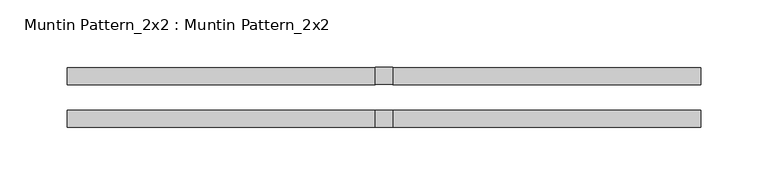
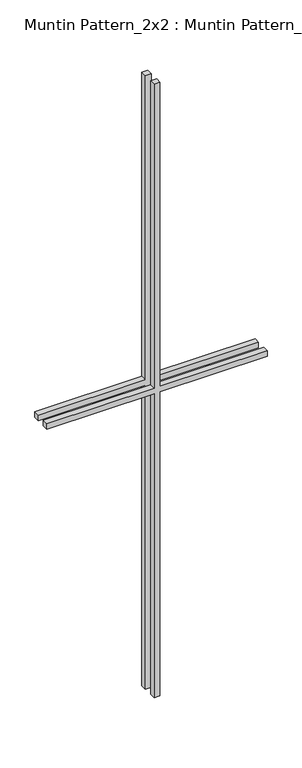
"""IFC4 building model written with IfcOpenShell, lengths in millimetres: proxy geometry, Muntin Pattern_2x2 : Muntin Pattern_2x2."""

from ifc_helpers import new_model, si_unit, frame, origin, place, context, project, spatial, polyline, outline, extrude, source, transform, mapped, element, save


def muntin_pattern_2x2_muntin_pattern_2x2_8031e6f6(model_context):
    return source(origin(), model_context, "Body", "SweptSolid", [
        extrude(outline(polyline([(698.5, -6.35), (698.5, -234.95), (685.8, -234.95), (685.8, -6.35), (0.0, -6.35), (0.0, 6.35), (685.8, 6.35), (685.8, 234.95), (698.5, 234.95), (698.5, 6.35), (1384.3, 6.35), (1384.3, -6.35), (698.5, -6.35)])), frame((0.0, 9.525, 0.0), z_axis=(0.0, 1.0, 0.0), x_axis=(0.0, 0.0, 1.0)), (0.0, 0.0, 1.0), 12.7),
        extrude(outline(polyline([(698.5, -6.35), (698.5, -234.95), (685.8, -234.95), (685.8, -6.35), (0.0, -6.35), (0.0, 6.35), (685.8, 6.35), (685.8, 234.95), (698.5, 234.95), (698.5, 6.35), (1384.3, 6.35), (1384.3, -6.35), (698.5, -6.35)])), frame((0.0, -22.225, 0.0), z_axis=(0.0, 1.0, 0.0), x_axis=(0.0, 0.0, 1.0)), (0.0, 0.0, 1.0), 12.7),
    ])


if __name__ == "__main__":
    model = new_model("IFC4")
    model_context = context("Model", 3, world=origin())
    ifc_project = project(units=[si_unit("LENGTHUNIT", "METRE", prefix="MILLI")], contexts=[model_context])
    site = spatial("IfcSite", under=ifc_project)
    building = spatial("IfcBuilding", under=site)
    placement = place(None, origin())
    muntin_pattern_2x2_muntin_pattern_2x2_shape = muntin_pattern_2x2_muntin_pattern_2x2_8031e6f6(model_context)
    element("IfcBuildingElementProxy", 1, Name="Muntin Pattern_2x2 : Muntin Pattern_2x2", ObjectType="Muntin Pattern_2x2 : Muntin Pattern_2x2", at=placement, inside=building, context=model_context, shape_type="MappedRepresentation", body=[
        mapped(muntin_pattern_2x2_muntin_pattern_2x2_shape, transform((0.0, 0.0, 0.0), x_axis=(1.0, 0.0, 0.0), y_axis=(0.0, 1.0, 0.0), z_axis=(0.0, 0.0, 1.0))),
    ])
    save(model, "model.ifc")

# Revit data of these elements
# Type "Muntin Pattern_2x2 : Muntin Pattern_2x2"
#   Width [instance default] = 4' - 0"
#   Thickness = 0' - 0 1/2"
#   Height [instance default] = 4' - 0"
#   Distance = 0' - 0 3/4"
#   Interior Material [instance default] = none
#   Exterior Material [instance default] = none
#   Default Elevation = 0
# Element 1 (IfcBuildingElementProxy, "Muntin Pattern_2x2 : Muntin Pattern_2x2")
#   Width = 1' - 6 1/2"
#   Height = 4' - 6 1/2"
#   Interior Material = Wood - Stained
#   Exterior Material = Clad - White
#   Materials on its faces: "Clad - White", "Wood - Stained"
# Materials
#   "Clad - White": class "Wood", colour RGB 242 242 238, transparency 0, Cost = 0
#   "Wood - Stained": class "Wood", colour RGB 224 178 126, transparency 0, Cost = 0
